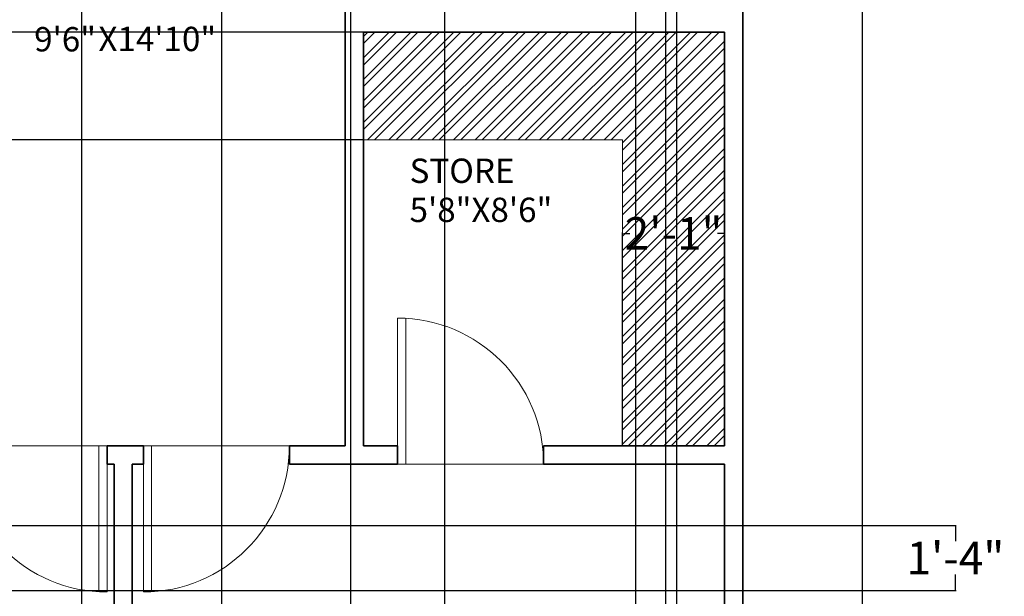
# Model space of a CAD drawing. Units: inches. Extents: x -438 to 102, y -60 to 1091.
# Tile 19 of 20: x -149 to 93, y 807 to 949. Entities that reach past the tile are written whole.
import ezdxf

# ---------------------------------------------------------------- set-up
doc = ezdxf.new("R2010")
doc.units = ezdxf.units.IN
doc.header["$MEASUREMENT"] = 0
for name, color, linetype, lineweight, true_color in [('A-ANNO-DIMS', 217, 'Continuous', 18, 0x93278f), ('A-DOOR', 30, 'Continuous', 18, 0xf26722), ('A-FLOR-CASE-PATT', 252, 'Continuous', 13, 0x939598), ('A-WALL', 2, 'Continuous', 35, 0xf1eb1f), ('C-PROP', 2, 'Continuous', 35, 0xf1eb1f)]:
    doc.layers.add(name, color=color, linetype=linetype, lineweight=lineweight, true_color=true_color)
doc.layers.add('A-AREA-IDEN', color=4, linetype='Continuous', lineweight=18)
doc.layers.add('A-FLOR-CASE', color=7, linetype='Continuous', lineweight=18)
doc.styles.get("Standard").update_dxf_attribs({"font": 'arial.ttf'})
doc.dimstyles.get("Standard").update_dxf_attribs({"dimtxt": 8, "dimasz": 0.18, "dimexe": 0.18, "dimexo": 0.0625, "dimgap": 0.09, "dimtad": 0, "dimtih": 1, "dimtoh": 1, "dimdec": 4, "dimzin": 0, "dimdsep": 46, "dimlunit": 3, "dimtxsty": 'Standard', "dimcen": 0.09, "dimadec": 0, "dimazin": 0, "dimtfac": 1, "dimtdec": 4, "dimtofl": 0, "dimtmove": 0, "dimatfit": 3, "dimfxl": 1, "dimtolj": 1, "dimtzin": 0, "dimarcsym": 0})

# ---------------------------------------------------------------- blocks, each defined once
blk = doc.blocks.new('*D5')
at = {"layer": 'A-ANNO-DIMS', "color": 0, "lineweight": -2, "transparency": 16777216}
for p, q in [((28.92, 1027), (58.42, 1027)), ((58.24, 1026.82), (58.24, 519.68)), ((58.24, 4.18), (58.24, 511.32)), ((28.92, 4), (58.42, 4))]:
    blk.add_line(p, q, dxfattribs=at)
at = {"layer": 'A-ANNO-DIMS', "color": 0, "transparency": 16777216}
for points in [[(58.21, 1026.82), (58.27, 1026.82), (58.24, 1027)], [(58.21, 4.18), (58.27, 4.18), (58.24, 4)]]:
    blk.add_solid(points, dxfattribs=at)
at = {"layer": 'Defpoints', "color": 0, "transparency": 16777216}
for p in [(28.85, 1027), (28.85, 4), (58.24, 4)]:
    blk.add_point(p, dxfattribs=at)
at = {"layer": 'A-ANNO-DIMS', "color": 0, "transparency": 16777216, "insert": (58.24, 515.5), "char_height": 8, "attachment_point": 5}
blk.add_mtext('\\A1;85\'-3.0000"', dxfattribs=at)
blk = doc.blocks.new('DOOR-SWING-36')
for p, q in [((-36, 0), (0, 0)), ((-2, 0), (-2, -36)), ((0, 0), (0, -36))]:
    blk.add_line(p, q)
blk.add_arc((0, 0), 36, 180, 270)
blk = doc.blocks.new('*D37')
at = {"layer": 'A-ANNO-DIMS', "color": 0, "lineweight": -2, "transparency": 16777216}
for p, q in [((-179.8, 234.94), (-179.8, 1079.58)), ((-179.62, 1079.4), (-176.98, 1079.4)), ((-134.26, 1079.4), (-136.9, 1079.4)), ((-134.08, 234.94), (-134.08, 1079.58))]:
    blk.add_line(p, q, dxfattribs=at)
at = {"layer": 'A-ANNO-DIMS', "color": 0, "transparency": 16777216}
for points in [[(-179.62, 1079.43), (-179.62, 1079.37), (-179.8, 1079.4)], [(-134.26, 1079.43), (-134.26, 1079.37), (-134.08, 1079.4)]]:
    blk.add_solid(points, dxfattribs=at)
at = {"layer": 'Defpoints', "color": 0, "transparency": 16777216}
for p in [(-134.08, 1079.4), (-179.8, 234.88), (-134.08, 234.88)]:
    blk.add_point(p, dxfattribs=at)
at = {"layer": 'A-ANNO-DIMS', "color": 0, "transparency": 16777216, "insert": (-156.94, 1079.4), "char_height": 8, "attachment_point": 5}
blk.add_mtext('\\A1;3\'-9 1/2"', dxfattribs=at)
blk = doc.blocks.new('*D43')
at = {"layer": 'A-ANNO-DIMS', "color": 0, "lineweight": -2, "transparency": 16777216}
for p, q in [((-0.78, 844.06), (-0.78, 896.58)), ((-0.6, 896.4), (1, 896.4)), ((24.17, 896.4), (22.58, 896.4)), ((24.35, 844.06), (24.35, 896.58))]:
    blk.add_line(p, q, dxfattribs=at)
at = {"layer": 'A-ANNO-DIMS', "color": 0, "transparency": 16777216}
for points in [[(-0.6, 896.43), (-0.6, 896.37), (-0.78, 896.4)], [(24.17, 896.43), (24.17, 896.37), (24.35, 896.4)]]:
    blk.add_solid(points, dxfattribs=at)
at = {"layer": 'Defpoints', "color": 0, "transparency": 16777216}
for p in [(24.35, 896.4), (-0.78, 844), (24.35, 844)]:
    blk.add_point(p, dxfattribs=at)
at = {"layer": 'A-ANNO-DIMS', "color": 0, "transparency": 16777216, "insert": (11.79, 896.4), "char_height": 8, "attachment_point": 5}
blk.add_mtext('\\A1;2\'-1"', dxfattribs=at)
blk = doc.blocks.new('*D44')
at = {"layer": 'A-ANNO-DIMS', "color": 0, "lineweight": -2, "transparency": 16777216}
for p, q in [((-64.71, 946), (-414.94, 946)), ((-414.76, 945.82), (-414.76, 936.94)), ((-414.76, 919.6), (-414.76, 928.48)), ((-64.71, 919.42), (-414.94, 919.42))]:
    blk.add_line(p, q, dxfattribs=at)
at = {"layer": 'A-ANNO-DIMS', "color": 0, "transparency": 16777216}
for points in [[(-414.79, 945.82), (-414.73, 945.82), (-414.76, 946)], [(-414.79, 919.6), (-414.73, 919.6), (-414.76, 919.42)]]:
    blk.add_solid(points, dxfattribs=at)
at = {"layer": 'Defpoints', "color": 0, "transparency": 16777216}
for p in [(-64.65, 946), (-414.76, 919.42), (-64.65, 919.42)]:
    blk.add_point(p, dxfattribs=at)
at = {"layer": 'A-ANNO-DIMS', "color": 0, "transparency": 16777216, "insert": (-414.76, 932.71), "char_height": 8, "attachment_point": 5}
blk.add_mtext('\\A1;2\'-2 1/2"', dxfattribs=at)
blk = doc.blocks.new('*D45')
at = {"layer": 'A-ANNO-DIMS', "color": 0, "lineweight": -2, "transparency": 16777216}
for p, q in [((-99.58, 615.92), (-99.58, 1079.58)), ((-99.4, 1079.4), (-59.27, 1079.4)), ((2.32, 1079.4), (-37.82, 1079.4)), ((2.5, 615.92), (2.5, 1079.58))]:
    blk.add_line(p, q, dxfattribs=at)
at = {"layer": 'A-ANNO-DIMS', "color": 0, "transparency": 16777216}
for points in [[(-99.4, 1079.43), (-99.4, 1079.37), (-99.58, 1079.4)], [(2.32, 1079.43), (2.32, 1079.37), (2.5, 1079.4)]]:
    blk.add_solid(points, dxfattribs=at)
at = {"layer": 'Defpoints', "color": 0, "transparency": 16777216}
for p in [(2.5, 1079.4), (-99.58, 615.86), (2.5, 615.86)]:
    blk.add_point(p, dxfattribs=at)
at = {"layer": 'A-ANNO-DIMS', "color": 0, "transparency": 16777216, "insert": (-48.54, 1079.4), "char_height": 8, "attachment_point": 5}
blk.add_mtext('\\A1;8\'-6"', dxfattribs=at)
blk = doc.blocks.new('*D47')
at = {"layer": 'A-ANNO-DIMS', "color": 0, "lineweight": -2, "transparency": 16777216}
for p, q in [((-67.74, 529.33), (-67.74, 1079.58)), ((-67.56, 1079.4), (-48.98, 1079.4)), ((9.73, 1079.4), (-8.85, 1079.4)), ((9.91, 529.33), (9.91, 1079.58))]:
    blk.add_line(p, q, dxfattribs=at)
at = {"layer": 'A-ANNO-DIMS', "color": 0, "transparency": 16777216}
for points in [[(-67.56, 1079.43), (-67.56, 1079.37), (-67.74, 1079.4)], [(9.73, 1079.43), (9.73, 1079.37), (9.91, 1079.4)]]:
    blk.add_solid(points, dxfattribs=at)
at = {"layer": 'Defpoints', "color": 0, "transparency": 16777216}
for p in [(9.91, 1079.4), (-67.74, 529.27), (9.91, 529.27)]:
    blk.add_point(p, dxfattribs=at)
at = {"layer": 'A-ANNO-DIMS', "color": 0, "transparency": 16777216, "insert": (-28.91, 1079.4), "char_height": 8, "attachment_point": 5}
blk.add_mtext('\\A1;6\'-5 1/2"', dxfattribs=at)
blk = doc.blocks.new('*D49')
at = {"layer": 'A-ANNO-DIMS', "color": 0, "lineweight": -2, "transparency": 16777216}
for p, q in [((-44.57, 339.86), (-44.57, 1079.58)), ((-44.39, 1079.4), (-26.89, 1079.4)), ((12.37, 1079.4), (-5.13, 1079.4)), ((12.55, 312.51), (12.55, 1079.58))]:
    blk.add_line(p, q, dxfattribs=at)
at = {"layer": 'A-ANNO-DIMS', "color": 0, "transparency": 16777216}
for points in [[(-44.39, 1079.43), (-44.39, 1079.37), (-44.57, 1079.4)], [(12.37, 1079.43), (12.37, 1079.37), (12.55, 1079.4)]]:
    blk.add_solid(points, dxfattribs=at)
at = {"layer": 'Defpoints', "color": 0, "transparency": 16777216}
for p in [(12.55, 1079.4), (-44.57, 339.79), (12.55, 312.44)]:
    blk.add_point(p, dxfattribs=at)
at = {"layer": 'A-ANNO-DIMS', "color": 0, "transparency": 16777216, "insert": (-16.01, 1079.4), "char_height": 8, "attachment_point": 5}
blk.add_mtext('\\A1;4\'-9"', dxfattribs=at)
blk = doc.blocks.new('*D54')
at = {"layer": 'A-ANNO-DIMS', "color": 0, "lineweight": -2, "transparency": 16777216}
for p, q in [((-214.3, 824.38), (81.43, 824.38)), ((81.25, 824.2), (81.25, 820.49)), ((81.25, 808.56), (81.25, 812.28)), ((-214.43, 808.38), (81.43, 808.38))]:
    blk.add_line(p, q, dxfattribs=at)
at = {"layer": 'A-ANNO-DIMS', "color": 0, "transparency": 16777216}
for points in [[(81.22, 824.2), (81.28, 824.2), (81.25, 824.38)], [(81.22, 808.56), (81.28, 808.56), (81.25, 808.38)]]:
    blk.add_solid(points, dxfattribs=at)
at = {"layer": 'Defpoints', "color": 0, "transparency": 16777216}
for p in [(-214.37, 824.38), (81.25, 824.38), (-214.49, 808.38)]:
    blk.add_point(p, dxfattribs=at)
at = {"layer": 'A-ANNO-DIMS', "color": 0, "transparency": 16777216, "insert": (81.25, 816.38), "char_height": 8, "attachment_point": 5}
blk.add_mtext('\\A1;1\'-4"', dxfattribs=at)

msp = doc.modelspace()

# ---------------------------------------------------------------- hatches: boundary and pattern name
at = {"layer": 'A-FLOR-CASE-PATT'}
h = msp.add_hatch(dxfattribs=at)
h.set_pattern_fill('ANSI32', color=256, scale=10)
h.set_pattern_definition([(45, (-842.8506, -448.43), (-2.6516504, 2.6516504), []), (45, (-841.083, -448.43), (-2.6516504, 2.6516504), [])])
h.paths.add_polyline_path([(24.35351, 945.99939), (-64.64649, 945.99939), (-64.64649, 919.41905), (-0.77524, 919.41905), (-0.77524, 843.99939), (24.35351, 843.99939)])

# ---------------------------------------------------------------- linework, layer by layer
at = {"layer": 'A-FLOR-CASE'}
for p, q in [((-64.64649, 919.41905), (-0.77524, 919.41905)), ((-0.77524, 919.41905), (-0.77524, 843.99939))]:
    msp.add_line(p, q, dxfattribs=at)
at = {"layer": 'A-WALL'}
for p, q in [((-69.14649, 956.94813), (-69.14649, 843.99939)), ((24.35351, 945.99939), (-64.64649, 945.99939)), ((-64.64649, 945.99939), (-64.64649, 843.99939)), ((24.35351, 843.99939), (24.35351, 945.99939)), ((-127.87208, 839.49939), (-127.87208, 843.99939)), ((-118.91198, 843.99939), (-127.87208, 843.99939)), ((-118.91198, 839.49939), (-118.91198, 843.99939)), ((-69.14649, 843.99939), (-82.91198, 843.99939)), ((-82.91198, 839.49939), (-82.91198, 843.99939)), ((-56.24437, 843.99939), (-64.64649, 843.99939)), ((-56.24437, 843.99939), (-56.24437, 839.49939)), ((24.35351, 843.99939), (-20.24437, 843.99939)), ((-20.24437, 843.99939), (-20.24437, 839.49939)), ((-126.14649, 839.49939), (-127.87208, 839.49939)), ((-126.14649, 665.49939), (-126.14649, 839.49939)), ((-121.64649, 665.49939), (-121.64649, 839.49939)), ((-118.91198, 839.49939), (-121.64649, 839.49939)), ((-56.24437, 839.49939), (-82.91198, 839.49939)), ((24.35351, 839.49939), (-20.24437, 839.49939)), ((24.35351, 665.49939), (24.35351, 839.49939))]:
    msp.add_line(p, q, dxfattribs=at)
at = {"layer": 'C-PROP'}
msp.add_line((28.85351, 3.99939), (28.85351, 1026.99939), dxfattribs=at)

# ---------------------------------------------------------------- block references
at = {"layer": 'A-DOOR', "rotation": 180}
msp.add_blockref('DOOR-SWING-36', (-56.24437, 839.49939), dxfattribs=at)
at = {"layer": 'A-DOOR'}
msp.add_blockref('DOOR-SWING-36', (-127.87208, 843.99939), dxfattribs=at)
at = {"layer": 'A-DOOR', "extrusion": (0, 0, -1), "zscale": -1}
msp.add_blockref('DOOR-SWING-36', (118.91198, 843.99939), dxfattribs=at)

# ---------------------------------------------------------------- texts
at = {"layer": 'A-AREA-IDEN'}
for s, p in [('9\'6"', (-145.82792, 941.24192)), ('X14\'10"', (-129.98814, 941.3148)), ('STORE', (-53.29026, 908.82788)), ('5\'8"X8\'6"', (-53.29026, 899.18941))]:
    msp.add_text(s, height=6, dxfattribs=at).set_placement(p)

# ---------------------------------------------------------------- dimensions: what is measured, and where the dimension line sits
at = {"layer": 'A-ANNO-DIMS'}
for base, p1, p2, picture, middle in [((-134.07948, 1079.39939), (-179.79585, 234.87846), (-134.07948, 234.87846), '*D37', (-156.93767, 1079.39939)), ((9.9115, 1079.39939), (-67.73982, 529.2655), (9.9115, 529.2655), '*D47', (-28.91416, 1079.39939)), ((2.49567, 1079.39939), (-99.58389, 615.85716), (2.49567, 615.85716), '*D45', (-48.54411, 1079.39939)), ((12.55306, 1079.39939), (-44.57214, 339.79496), (12.55306, 312.44261), '*D49', (-16.00954, 1079.39939)), ((24.35351, 896.39939), (-0.77524, 843.99939), (24.35351, 843.99939), '*D43', (11.78914, 896.39939))]:
    dim = msp.add_linear_dim(base=base, p1=p1, p2=p2, dimstyle='Standard', override={"dimdec": 1, "dimlfac": 1, "dimrnd": 0, "dimzin": 1, "dimdsep": 46, "dimlunit": 4, "dimfrac": 2}, dxfattribs=at)
    dim.commit()
    dim.dimension.update_dxf_attribs({"geometry": picture, "text_midpoint": middle})
for base, p1, p2, override, picture, middle in [((58.24207, 3.99939), (28.85351, 1026.99939), (28.85351, 3.99939), {"dimclrd": 0, "dimclre": 0, "dimclrt": 0}, '*D5', (58.24207, 515.49939)), ((-414.76009, 919.41905), (-64.64649, 945.99939), (-64.64649, 919.41905), {"dimdec": 1, "dimlfac": 1, "dimrnd": 0, "dimzin": 1, "dimdsep": 46, "dimlunit": 4, "dimfrac": 2}, '*D44', (-414.76009, 932.70922)), ((81.25351, 824.37939), (-214.49234, 808.38394), (-214.3672, 824.37939), {"dimdec": 1, "dimlfac": 1, "dimrnd": 0, "dimzin": 1, "dimdsep": 46, "dimlunit": 4, "dimfrac": 2}, '*D54', (81.25351, 816.38167))]:
    dim = msp.add_linear_dim(base=base, p1=p1, p2=p2, angle=90, dimstyle='Standard', override=override, dxfattribs=at)
    dim.commit()
    dim.dimension.update_dxf_attribs({"geometry": picture, "text_midpoint": middle})

doc.saveas('drawing.dxf')
